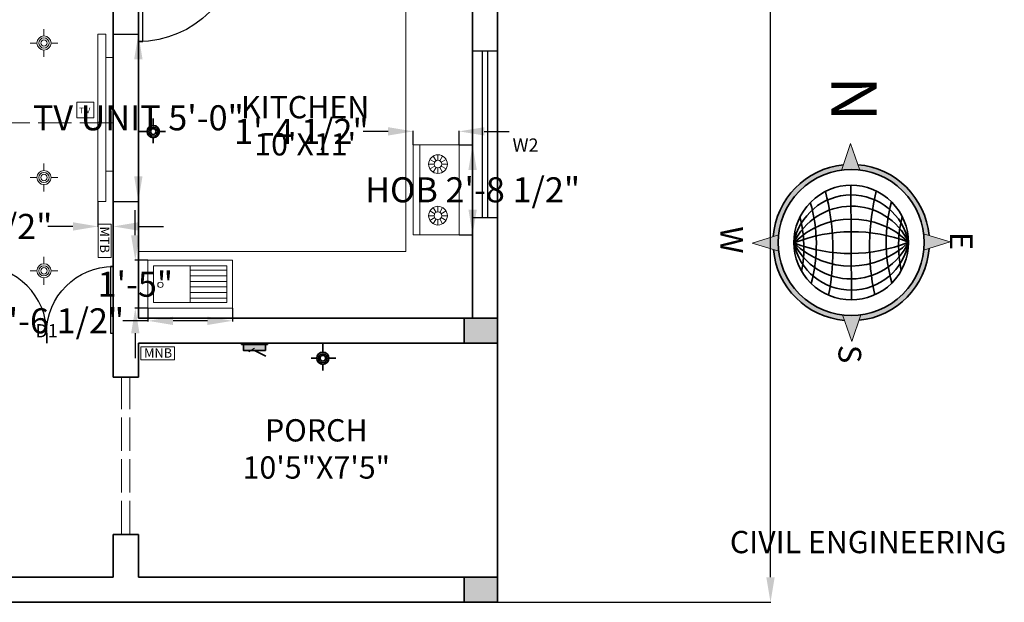
# Model space of a CAD drawing. Units: inches. Extents: x 68 to 1275, y 90 to 1276.
# Tile 5 of 6: x 916 to 1270, y 603 to 813. Entities that reach past the tile are written whole.
import ezdxf

# ---------------------------------------------------------------- set-up
doc = ezdxf.new("R2010")
doc.units = ezdxf.units.IN
doc.header["$MEASUREMENT"] = 0
doc.linetypes.add('ACAD_ISO02W100', pattern=[15, 12, -3])
for name, color, linetype, lineweight in [('A -Elec', 6, 'Continuous', 18), ('A- WALL', 7, 'Continuous', 35), ('A-ANNO-SYMB', 7, 'Continuous', 18), ('A-ANNO-TEXT', 7, 'Continuous', 18), ('A-AREA-IDEN', 7, 'Continuous', 18), ('A-EQPM', 9, 'Continuous', 18), ('A-FLOR-FIXT', 9, 'Continuous', 18), ('A-FLOR-OVHD', 8, 'ACAD_ISO02W100', 13), ('A-TEXT', 7, 'Continuous', 9), ('A-WALL', 7, 'Continuous', 35), ('COLUMN', 150, 'Continuous', 35), ('DIM', 2, 'Continuous', 18), ('DOOR', 15, 'Continuous', 25), ('E-LITE', 6, 'Continuous', 18), ('E-POWR', 1, 'Continuous', 18), ('E-REFR', 8, 'ACAD_ISO02W100', 13), ('Elec', 1, 'Continuous', 35), ('FURN', 163, 'Continuous', 18), ('WINDOW', 17, 'Continuous', 18)]:
    doc.layers.add(name, color=color, linetype=linetype, lineweight=lineweight)
doc.styles.get("Standard").update_dxf_attribs({"font": 'arial.ttf'})
doc.dimstyles.get("Standard").update_dxf_attribs({"dimtxt": 9, "dimasz": 9, "dimexe": 0.18, "dimexo": 0.0625, "dimgap": 0.09, "dimtad": 0, "dimtih": 1, "dimtoh": 1, "dimdec": 1, "dimzin": 0, "dimdsep": 46, "dimlunit": 3, "dimtxsty": 'Standard', "dimcen": 0.09, "dimadec": 0, "dimazin": 0, "dimtfac": 1, "dimtdec": 1, "dimtofl": 0, "dimtmove": 0, "dimatfit": 3, "dimfxl": 1, "dimtolj": 1, "dimtzin": 0, "dimarcsym": 0})

# ---------------------------------------------------------------- blocks, each defined once
blk = doc.blocks.new('*U2')
for p, q in [((0, 0), (-1e-16, -5.999999999999999)), ((40, -6e-16), (40, -6))]:
    blk.add_line(p, q)
blk.add_lwpolyline([(0, 0), (5.6e-15, 40), (1.750000000000007, 40), (1.749999999999998, -7e-16)], close=True)
blk.add_arc((0, 0), 40, 0, 90)
blk = doc.blocks.new('W')
at = {"layer": 'DOOR'}
for p, q in [((91.83571953581463, 414.9514425754601), (100.8357195358146, 414.9514425754601)), ((91.83571953581463, 354.9514425754601), (91.8357195358146, 414.9514425754601)), ((95.33571953581462, 354.9514425754601), (95.33571953581462, 414.9514425754601)), ((97.33571953581463, 354.9514425754601), (97.33571953581463, 414.9514425754601)), ((100.8357195358146, 414.9514425754601), (100.8357195358146, 354.9514425754601)), ((100.8357195358146, 354.9514425754601), (91.83571953581463, 354.9514425754601))]:
    blk.add_line(p, q, dxfattribs=at)
blk = doc.blocks.new('C')
h = blk.add_hatch(color=256)
h.dxf.hatch_style = 1
h.paths.add_polyline_path([(745.8101109123093, 845.9819968167334), (745.8101109123093, 857.9819968167335), (736.8101109123093, 857.9819968167335), (736.8101109123093, 845.9819968167334)])
for p, q in [((745.8101109123093, 857.9819968167335), (736.8101109123093, 857.9819968167335)), ((736.8101109123093, 857.9819968167335), (736.8101109123093, 845.9819968167334)), ((745.8101109123093, 845.9819968167334), (745.8101109123093, 857.9819968167335)), ((736.8101109123093, 845.9819968167334), (745.8101109123093, 845.9819968167334))]:
    blk.add_line(p, q)
blk = doc.blocks.new('TV')
for points in [[(1846.6449218592, 1133.158042881319), (1849.487420558524, 1133.158042881319), (1849.487420558524, 1073.144323226678), (1846.6449218592, 1073.144323226678)], [(1846.6449218592, 1122.373694788675), (1843.999810833538, 1122.373694788675), (1843.999810833538, 1081.482214013656), (1846.6449218592, 1081.482214013656)]]:
    blk.add_lwpolyline(points, close=True)
blk = doc.blocks.new('DIRECTION')
at = {"layer": 'DIM', "ltscale": 35}
h = blk.add_hatch(color=256, dxfattribs=at)
h.dxf.hatch_style = 1
edge = h.paths.add_edge_path()
edge.add_line((2597.24832190935, 2408.269559539512), (2601.856533232682, 2393.62299110183))
edge.add_ellipse((2597.639423319343, 2353.481842285464), major_axis=(28.54028595385228, -28.5402859538523), ratio=0.9999999999827393, start_angle=129.0026750704451, end_angle=135.4089982327699)
edge.add_ellipse((2597.639423319602, 2353.481842285464), major_axis=(-28.54028595291803, -28.54028595291801), ratio=0.999999999985297, start_angle=225.4089982331304, end_angle=231.8159173823239)
edge.add_line((2592.849261358955, 2393.558645959323), (2597.248321909339, 2408.269559539583))
h = blk.add_hatch(color=256, dxfattribs=at)
h.dxf.hatch_style = 1
edge = h.paths.add_edge_path()
edge.add_line((2637.716337406115, 2348.692604170624), (2640.725786551334, 2349.752367405582))
edge.add_ellipse((2597.639423319343, 2353.481842285464), major_axis=(-30.58057945317442, -30.5805794531744), ratio=0.9999999999976388, start_angle=50.166226554127775, end_angle=130.0529151095595, ccw=False)
edge.add_line((2601.533664809112, 2310.41005845266), (2602.42916840349, 2313.404988786752))
edge.add_ellipse((2597.639423319343, 2353.481842285464), major_axis=(-28.54028595136435, -28.54028595136432), ratio=0.9999999999994514, start_angle=51.81532139532596, end_angle=128.185403391547)
edge = h.paths.add_edge_path()
edge.add_line((2593.421895860988, 2313.340737337358), (2594.360152675466, 2310.358877830749))
edge.add_ellipse((2597.639423319343, 2353.481842285464), major_axis=(-30.58057945314276, -30.58057945314273), ratio=0.9999999999967295, start_angle=320.7650813562228, end_angle=400.6513322142664, ccw=False)
edge.add_line((2554.610693956437, 2349.137635932355), (2557.634965847779, 2348.12094433685))
edge.add_ellipse((2597.639423319343, 2353.481842285464), major_axis=(28.54028595137265, -28.54028595137269), ratio=0.9999999999998977, start_angle=232.6325930742551, end_angle=309.0020790836279)
edge = h.paths.add_edge_path()
edge.add_line((2557.562509232831, 2358.271080400352), (2554.553060087694, 2357.211317165394))
edge.add_ellipse((2597.639423319343, 2353.481842285464), major_axis=(-30.58057945310715, -30.58057945310715), ratio=0.9999999999999497, start_angle=230.1666642515818, end_angle=310.0529151095499, ccw=False)
edge.add_line((2593.744852793148, 2396.553596367937), (2592.849261358943, 2393.558645959394))
edge.add_ellipse((2597.639423319343, 2353.481842285464), major_axis=(28.5402859513619, -28.54028595136188), ratio=0.9999999999987931, start_angle=141.8159173820852, end_angle=218.1854033915469)
edge = h.paths.add_edge_path()
edge.add_line((2601.85653323267, 2393.622991101876), (2600.918364535997, 2396.604831790109))
edge.add_ellipse((2597.639423319343, 2353.481842285464), major_axis=(-30.58057945312165, -30.58057945312163), ratio=0.9999999999985156, start_angle=140.765081356223, end_angle=220.6517699116423, ccw=False)
edge.add_line((2640.668152682508, 2357.826048638621), (2637.643880791167, 2358.842740234127))
edge.add_ellipse((2597.639423319343, 2353.481842285464), major_axis=(28.54028595137743, -28.54028595137745), ratio=0.9999999999999049, start_angle=52.63259307425506, end_angle=129.0026750705646)
h = blk.add_hatch(color=256, dxfattribs=at)
h.dxf.hatch_style = 1
edge = h.paths.add_edge_path()
edge.add_ellipse((2597.639423319343, 2353.481842285464), major_axis=(-28.54028595210723, -28.54028595210721), ratio=0.999999999994473, start_angle=308.1854033915466, end_angle=322.6325930742547)
edge.add_line((2557.634965847779, 2348.120944336826), (2542.851706063651, 2353.090740875343))
edge.add_line((2542.851706063651, 2353.090740875343), (2557.562509232831, 2358.271080400328))
h = blk.add_hatch(color=256, dxfattribs=at)
h.dxf.hatch_style = 1
edge = h.paths.add_edge_path()
edge.add_line((2637.643880791167, 2358.84274023415), (2652.427140575295, 2353.87294369554))
edge.add_line((2652.427140575295, 2353.87294369554), (2637.716337406114, 2348.692604170648))
edge.add_ellipse((2597.639423319343, 2353.481842285464), major_axis=(-28.54028595030189, -28.54028595030183), ratio=0.9999999999925798, start_angle=128.1854033915468, end_angle=142.632593074255)
h = blk.add_hatch(color=256, dxfattribs=at)
h.dxf.hatch_style = 1
edge = h.paths.add_edge_path()
edge.add_line((2602.42916840349, 2313.404988786869), (2598.030524729594, 2298.694125031464))
edge.add_line((2598.030524729594, 2298.69412503137), (2593.421895860988, 2313.340737337334))
edge.add_ellipse((2597.639423319602, 2353.481842285464), major_axis=(28.54028595190623, -28.54028595190623), ratio=0.9999999999939888, start_angle=-50.99792091661058, end_angle=-44.59100176735014)
edge.add_ellipse((2597.639423319343, 2353.481842285464), major_axis=(-28.54028595335771, -28.54028595335769), ratio=0.9999999999832972, start_angle=45.40899823301023, end_angle=51.81532139544526)
at = {"layer": 'A- WALL', "ltscale": 35}
blk.add_line((2629.34444276032, 2353.708168156072), (2565.934403878626, 2353.255516414717), dxfattribs=at)
at = {"layer": 'A- WALL', "ltscale": 35, "extrusion": (0, 0, -1)}
for centre, major_axis, ratio, start_param, end_param in [((2597.639423319343, 2353.481842285418), (-30.58057945312132, -30.58057945312131), 0.9999999999987959, 0.8717410831091346, 2.266019187658509), ((2597.639423319343, 2353.481842285418), (28.5402859514277, -28.5402859514277), 0.9999999999973692, 3.919852451189786, 10.20303775836937), ((2597.639423319343, 2353.481842285418), (-30.58057945314268, -30.58057945314266), 0.9999999999988618, 2.432085421867908, 3.826371165679486), ((2597.639423319343, 2353.481842285418), (22.41940544614458, -22.41940544614459), 0.999999999999132, 3.919852451188904, 10.20303775836849), ((2603.542187591361, 2353.523989522555), (22.80466912504525, -22.80466912504527), 0.9999999999934116, 0.9623333078138184, 3.735775406983438), ((2612.505423052941, 2353.587989301701), (-24.76160024723522, -24.76160024723521), 0.9999999999992525, -0.3540869259178678, 1.910602987118144), ((2629.757673802409, 2353.71112763613), (-31.9131967420592, -31.91319674205919), 0.9999999999985343, -0.0006610730671919, 1.55718066820378), ((2599.182585971628, 2445.662182832683), (46.62855256632114, -46.62855256632116), 0.9999999999994293, 0.5735918910566035, 1.030682691728694), ((2678.031679859687, 2354.055802032412), (-61.10857846222063, -61.10857846222057), 0.999999999998412, 0.4026080436482158, 1.153909784551204), ((2517.246998575127, 2352.907900606915), (61.1085784622124, -61.10857846221246), 0.9999999999999429, 5.114997024032398, 5.866298764935286), ((2565.521005037576, 2353.252518252051), (-31.91319674206676, -31.91319674206674), 0.9999999999991755, 3.140929813589933, 4.698771554849301), ((2591.736490906592, 2353.439704278876), (-22.80466912498845, -22.80466912498845), 0.9999999999995747, 2.533131401603469, 5.306573500773075), ((2582.773255331945, 2353.375720337799), (-24.76160024727029, -24.76160024727029), 0.9999999999990459, 2.78750749467719, 5.052197407698938), ((2597.115156409695, 2454.394147896003), (-57.71452300102988, -57.71452300102983), 0.9999999999994852, -1.068719002289636, -0.5124677756952505), ((2597.639423319343, 2353.481842285418), (-30.58057945309982, -30.5805794530998), 0.9999999999997768, -0.7094995924610965, 0.6847785120890495), ((2597.639423319343, 2353.481842285418), (-30.58057945319512, -30.58057945319512), 0.9999999999962719, 4.013333736700001, 5.407619480506816), ((2601.743533004009, 2216.179397968859), (-89.95633825845869, -89.95633825845869), 0.9999999999989515, 2.098588931419211, 2.554035810148795), ((2598.555858798734, 2252.572336165166), (-57.71452300096218, -57.71452300096211), 0.9999999999999362, 2.068987370893696, 2.625238597487658)]:
    blk.add_ellipse(centre, major_axis=major_axis, ratio=ratio, start_param=start_param, end_param=end_param, dxfattribs=at)
at = {"layer": 'A- WALL', "ltscale": 35, "extrusion": (0, 0, -0.9999999999999998)}
for centre, major_axis, ratio, start_param, end_param in [((2599.782951195766, 2490.828885281749), (89.95633825820524, -89.95633825820524), 0.9999999999996148, 0.5732801118446276, 1.028726990569549), ((2600.498417980858, 2261.332926481243), (-46.62855256648622, -46.6285525664862), 0.9999999999990784, 2.096633230266009, 2.553724030937174)]:
    blk.add_ellipse(centre, major_axis=major_axis, ratio=ratio, start_param=start_param, end_param=end_param, dxfattribs=at)
at = {"layer": 'DIM', "ltscale": 35}
for p, q in [((2597.24832190935, 2408.269559539489), (2592.827539238222, 2393.486004940269)), ((2597.24832190935, 2408.269559539489), (2601.879338537261, 2393.550507565663)), ((2542.851706063651, 2353.090740875319), (2557.656003696302, 2358.30400403195)), ((2652.427140575295, 2353.872943695493), (2637.549925830003, 2358.874325760384)), ((2542.851706063651, 2353.090740875319), (2557.728920809025, 2348.089358810546)), ((2652.427140575295, 2353.872943695493), (2637.622842942642, 2348.659680538956)), ((2598.030524729594, 2298.694125031323), (2593.399138912629, 2313.41306084311)), ((2598.030524729594, 2298.694125031323), (2602.450936591041, 2313.477790510296))]:
    blk.add_line(p, q, dxfattribs=at)
at = {"layer": 'A-TEXT', "char_height": 13.629465702112, "width": 273.2349075094469, "attachment_point": 2}
for s, insert in [('{\\fTimes New Roman|b0|i0|c0|p18;\\H0.9233x;E}', (2596.77738151443, 2420.65579489876)), ('{\\fTimes New Roman|b0|i0|c0|p18;\\H0.9233x;S}', (2659.361945474433, 2358.999040747372)), ('{\\fTimes New Roman|b0|i0|c0|p18;\\H0.9233x;W}', (2596.170612003199, 2293.619718441945))]:
    blk.add_mtext(s, dxfattribs=dict(at, insert=insert))
at = {"layer": 'A-TEXT', "insert": (2518.058106811495, 2342.398918831673), "char_height": 27.25893140422401, "width": 546.4698150188938, "attachment_point": 2, "rotation": 179.99999999999997}
blk.add_mtext('{\\fTimes New Roman|b0|i0|c0|p18;\\H0.9233x;N}', dxfattribs=at)
blk = doc.blocks.new('*U28')
blk.add_line((0, 1), (0, -1))
blk = doc.blocks.new('*U29')
at = {"layer": 'FURN', "transparency": 16777216}
blk.add_blockref('*U28', (1741.424228826588, 1059.606151326937), dxfattribs=at)
for p, rotation in [((1739.058647081696, 1057.240569582045), 90), ((1739.375574940783, 1058.423360454491), 59.99999999999999), ((1740.241437954142, 1059.28922346785), 30), ((1742.607019699035, 1059.28922346785), 330.0000000000001), ((1743.472882712394, 1058.423360454491), 300), ((1743.789810571481, 1057.240569582045), 270), ((1739.375574940783, 1056.057778709598), 120), ((1740.241437954142, 1055.191915696239), 150), ((1741.424228826588, 1054.874987837152), 180), ((1742.607019699035, 1055.191915696239), 210), ((1743.472882712394, 1056.057778709598), 240)]:
    blk.add_blockref('*U28', p, dxfattribs=dict(at, rotation=rotation))
blk = doc.blocks.new('*U30')
blk.add_line((0, 1), (0, -1))
blk = doc.blocks.new('*U31')
at = {"layer": 'FURN', "transparency": 16777216}
blk.add_blockref('*U30', (1741.424228826588, 1059.606151326937), dxfattribs=at)
for p, rotation in [((1739.058647081696, 1057.240569582045), 90), ((1739.375574940783, 1058.423360454491), 59.99999999999999), ((1740.241437954142, 1059.28922346785), 30), ((1742.607019699035, 1059.28922346785), 330.0000000000001), ((1743.472882712394, 1058.423360454491), 300), ((1743.789810571481, 1057.240569582045), 270), ((1739.375574940783, 1056.057778709598), 120), ((1740.241437954142, 1055.191915696239), 150), ((1741.424228826588, 1054.874987837152), 180), ((1742.607019699035, 1055.191915696239), 210), ((1743.472882712394, 1056.057778709598), 240)]:
    blk.add_blockref('*U30', p, dxfattribs=dict(at, rotation=rotation))
blk = doc.blocks.new('GAS')
at = {"layer": 'FURN'}
blk.add_line((1734.581424903461, 1063.742262082391), (1766.852210475836, 1063.742262082391), dxfattribs=at)
blk.add_lwpolyline([(1734.581424903461, 1066.149269907321), (1766.852210475836, 1066.149269907321), (1766.852210475836, 1049.6497415827), (1734.581424903461, 1049.6497415827)], close=True, dxfattribs=at)
for centre, radius in [((1741.424228826588, 1057.240569582045), 3.365581744892551), ((1759.93108495299, 1057.240569582045), 3.365581744892551), ((1741.424228826588, 1057.240569582045), 1.365581744892551), ((1759.93108495299, 1057.240569582045), 1.365581744892551)]:
    blk.add_circle(centre, radius, dxfattribs=at)
for name, p in [('*U29', (0, 0)), ('*U31', (18.50685612640154, 0))]:
    blk.add_blockref(name, p, dxfattribs=at)
blk = doc.blocks.new('SINK')
for p, q in [((1691.404714224582, 1155.421202546591), (1708.596639589884, 1155.421202546591)), ((1708.596639589884, 1155.421202546591), (1708.596639589884, 1125.071391182841)), ((1693.404714224582, 1140.246296864716), (1706.596639589884, 1140.246296864716)), ((1695.009100856844, 1140.246296864716), (1695.009100856844, 1127.071391182841)), ((1697.009100856844, 1140.246296864716), (1697.009100856844, 1127.071391182841)), ((1699.009100856844, 1140.246296864716), (1699.009100856844, 1127.071391182841)), ((1701.009100856844, 1140.246296864716), (1701.009100856844, 1127.071391182841)), ((1703.009100856844, 1140.246296864716), (1703.009100856844, 1127.071391182841)), ((1705.009100856844, 1140.246296864716), (1705.009100856844, 1127.071391182841))]:
    blk.add_line(p, q)
for points in [[(1691.404714224582, 1155.421202546591), (1708.596639589884, 1155.421202546591), (1708.596639589884, 1125.071391182841), (1691.404714224582, 1125.071391182841)], [(1693.404714224582, 1153.421202546591), (1706.596639589884, 1153.421202546591), (1706.596639589884, 1127.071391182841), (1693.404714224582, 1127.071391182841)]]:
    blk.add_lwpolyline(points, close=True)
blk.add_circle((1699.780821048727, 1150.931238269399), 0.9650765021387996)
blk = doc.blocks.new('splight')
at = {"layer": 'Elec'}
for p, q in [((4618.165493646445, 527.1595508907546), (4627.57380882646, 527.1595508907546)), ((4622.869651236451, 527.1595508907546), (4622.869651236451, 523.8688723625129)), ((4620.576181531769, 521.5754026578305), (4618.052205676129, 521.5754026578305)), ((4622.869651236451, 519.2819329531479), (4622.869651236451, 517.0346704452847)), ((4625.163120941137, 521.5754026578305), (4627.232633020232, 521.5754026578305))]:
    blk.add_line(p, q, dxfattribs=at)
for radius in [2.293469704682637, 1.668469704682639, 1.043469704682639]:
    blk.add_circle((4622.869651236451, 521.5754026578305), radius, dxfattribs=at)
blk = doc.blocks.new('CIELING')
at = {"layer": 'A -Elec'}
for p, q in [((1070.869500591183, -8395.655580837194), (1070.869500591183, -8391.485789029257)), ((1066.613971407157, -8399.911110021205), (1062.44417959922, -8399.911110021205)), ((1070.869500591183, -8408.33643101315), (1070.869500591183, -8404.166639205214)), ((1075.125029775208, -8399.911110021205), (1079.294821583145, -8399.911110021205))]:
    blk.add_line(p, q, dxfattribs=at)
for radius in [4.255529184009533, 3.095842734009534, 1.936156284009533]:
    blk.add_circle((1070.869500591183, -8399.911110021205), radius, dxfattribs=at)
blk = doc.blocks.new('elec box')
at = {"layer": 'Elec'}
blk.add_hatch(color=256, dxfattribs=at).paths.add_polyline_path([(3828.234962737587, 599.2881263179643), (3828.234962737587, 594.7881263179643), (3844.734962737589, 594.7881263179643), (3844.734962737589, 599.2881263179643)])
for p, q in [((3836.484962737588, 599.2881263179643), (3828.066979685118, 603.4529863194257)), ((3846.10280273742, 594.7881263179643), (3826.830962060027, 594.7881263179643)), ((3826.830962060027, 594.7881263179643), (3826.830962060027, 593.8893551118417)), ((3826.830962060027, 593.8893551118417), (3846.10280273742, 593.8893551118417)), ((3846.10280273742, 593.8893551118417), (3846.10280273742, 594.7881263179643))]:
    blk.add_line(p, q, dxfattribs=at)
blk.add_lwpolyline([(3828.234962737587, 594.7881263179643), (3828.234962737587, 599.2881263179643), (3844.734962737589, 599.2881263179643), (3844.734962737589, 594.7881263179643), (3828.234962737587, 594.7881263179643)], dxfattribs=at)
blk = doc.blocks.new('SWITCHBOARD-ONE-WAY')
blk.add_line((4.634474659967281, 1.72886330620372), (6.643170124125163, 3.124132868275296))
at = {"xscale": 0.480395109260985, "yscale": 0.480395109260985, "zscale": 0.480395109260985}
blk.add_blockref('elec box', (-1838.391242964724, -285.3017071861163), dxfattribs=at)
blk = doc.blocks.new('TV-POINT')
blk.add_lwpolyline([(2.2128117507e-06, 5.568118865895371), (6.100736396045249, 5.568118865895371), (6.100736396045249, -7.01044664311e-05), (2.2128117507e-06, -7.01044664311e-05)], close=True)
at = {"transparency": 33554676}
blk.add_lwpolyline([(2.2128117507e-06, 5.568118865895371), (6.100736396045249, 5.568118865895371), (6.100736396045249, -7.01044664311e-05), (2.2128117507e-06, -7.01044664311e-05)], close=True, dxfattribs=at)
at = {"insert": (0.8393167226115565, 3.647168321161302), "char_height": 2.003474701485161, "attachment_point": 1}
blk.add_mtext('T.V ', dxfattribs=at)
at = {"transparency": 33554676, "insert": (0.8393167226115565, 3.647168321161302), "char_height": 2.003474701485161, "attachment_point": 1}
blk.add_mtext('T.V ', dxfattribs=at)
blk = doc.blocks.new('MAIN-BOARD')
blk.add_lwpolyline([(0.0004361200251424, 4.703133274055858), (12.06279134155943, 4.703133274055858), (12.06279134155943, 0.0003298403245253), (0.0004361200251424, 0.0003298403245253)], close=True)
blk.add_text('MNB', height=3.362765764821897).set_placement((1.14402048200327, 0.7969751531460361))
blk = doc.blocks.new('METER-BOARD')
blk.add_lwpolyline([(0.0004361200251424, 4.702354804303354), (12.06279134155943, 4.702354804303354), (12.06279134155943, -0.0004486294279786), (0.0004361200251424, -0.0004486294279786)], close=True)
blk.add_text('MTB', height=3.362765764821897).set_placement((0.8731259797250459, 0.6934873088445102))
blk = doc.blocks.new('*D67')
at = {"layer": 'Defpoints', "color": 0, "transparency": 16777216}
for p in [(949.6262836938411, 807.4231390285687), (949.6262836938411, 747.4094193739274), (958.6283416420378, 747.4094193739274)]:
    blk.add_point(p, dxfattribs=at)
at = {"layer": 'DIM', "color": 0, "lineweight": -2, "transparency": 16777216}
for p, q in [((949.6887836938411, 807.4231390285687), (958.8083416420376, 807.4231390285687)), ((958.6283416420378, 798.4231390285688), (958.6283416420378, 782.1014360907435)), ((958.6283416420378, 756.4094193739274), (958.6283416420378, 772.731122311753)), ((949.6887836938411, 747.4094193739274), (958.8083416420378, 747.4094193739274))]:
    blk.add_line(p, q, dxfattribs=at)
at = {"layer": 'DIM', "color": 0, "transparency": 16777216}
for points in [[(957.1283416420378, 798.4231390285688), (960.1283416420378, 798.4231390285688), (958.6283416420378, 807.4231390285687)], [(957.1283416420378, 756.4094193739274), (960.1283416420379, 756.4094193739274), (958.6283416420378, 747.4094193739274)]]:
    blk.add_solid(points, dxfattribs=at)
at = {"layer": 'DIM', "color": 0, "transparency": 16777216, "insert": (958.6283416420378, 777.4162792012476), "char_height": 9, "attachment_point": 5}
blk.add_mtext('\\A1;TV UNIT 5\'-0"', dxfattribs=at)
blk = doc.blocks.new('*D68')
at = {"layer": 'Defpoints', "color": 0, "transparency": 16777216}
for p in [(944.1386739688546, 747.4094193739272), (949.6262836938406, 747.4094193739272), (944.1386739688546, 738.407361425731)]:
    blk.add_point(p, dxfattribs=at)
at = {"layer": 'DIM', "color": 0, "lineweight": -2, "transparency": 16777216}
for p, q in [((944.1386739688546, 747.3469193739272), (944.1386739688546, 738.2273614257311)), ((949.6262836938406, 747.3469193739272), (949.6262836938406, 738.2273614257311)), ((935.1386739688546, 738.407361425731), (926.1386739688546, 738.407361425731)), ((958.6262836938406, 738.407361425731), (967.6262836938406, 738.407361425731))]:
    blk.add_line(p, q, dxfattribs=at)
at = {"layer": 'DIM', "color": 0, "transparency": 16777216}
for points in [[(935.1386739688546, 739.9073614257311), (935.1386739688546, 736.9073614257311), (944.1386739688546, 738.407361425731)], [(958.6262836938406, 739.9073614257311), (958.6262836938406, 736.9073614257311), (949.6262836938406, 738.407361425731)]]:
    blk.add_solid(points, dxfattribs=at)
at = {"layer": 'DIM', "color": 0, "transparency": 16777216, "insert": (903.6008567792229, 738.407361425731), "char_height": 9, "attachment_point": 5}
blk.add_mtext('\\A1;0\'-5 1/2"', dxfattribs=at)
blk = doc.blocks.new('*D69')
at = {"layer": 'Defpoints', "color": 0, "transparency": 16777216}
for p in [(962.0814133719534, 709.0733946794592), (992.4312247357036, 709.0733946794592), (962.0814133719534, 704.5209229748966)]:
    blk.add_point(p, dxfattribs=at)
at = {"layer": 'DIM', "color": 0, "lineweight": -2, "transparency": 16777216}
for p, q in [((962.0814133719534, 709.010894679459), (962.0814133719534, 704.3409229748966)), ((992.4312247357036, 709.010894679459), (992.4312247357036, 704.3409229748966)), ((962.0814133719534, 704.5209229748966), (953.0814133719534, 704.5209229748966)), ((983.4312247357036, 704.5209229748966), (971.0814133719534, 704.5209229748966))]:
    blk.add_line(p, q, dxfattribs=at)
at = {"layer": 'DIM', "color": 0, "transparency": 16777216}
for points in [[(971.0814133719534, 706.0209229748966), (971.0814133719534, 703.0209229748966), (962.0814133719534, 704.5209229748966)], [(983.4312247357036, 706.0209229748966), (983.4312247357036, 703.0209229748966), (992.4312247357036, 704.5209229748966)]]:
    blk.add_solid(points, dxfattribs=at)
at = {"layer": 'DIM', "color": 0, "transparency": 16777216, "insert": (914.1459154183381, 704.5209229748966), "char_height": 9, "attachment_point": 5}
blk.add_mtext('\\A1;SINK 2\'-6 1/2"', dxfattribs=at)
blk = doc.blocks.new('*D70')
at = {"layer": 'Defpoints', "color": 0, "transparency": 16777216}
for p in [(957.5289416673916, 726.2653200447614), (962.0814133719539, 726.2653200447614), (962.0814133719539, 709.0733946794594)]:
    blk.add_point(p, dxfattribs=at)
at = {"layer": 'DIM', "color": 0, "lineweight": -2, "transparency": 16777216}
for p, q in [((957.5289416673916, 735.2653200447614), (957.5289416673916, 744.2653200447614)), ((962.0189133719538, 726.2653200447614), (957.3489416673917, 726.2653200447614)), ((962.0189133719538, 709.0733946794594), (957.3489416673917, 709.0733946794594)), ((957.5289416673916, 700.0733946794594), (957.5289416673916, 691.0733946794594))]:
    blk.add_line(p, q, dxfattribs=at)
at = {"layer": 'DIM', "color": 0, "transparency": 16777216}
for points in [[(956.0289416673917, 735.2653200447614), (959.0289416673916, 735.2653200447614), (957.5289416673916, 726.2653200447614)], [(956.0289416673917, 700.0733946794594), (959.0289416673916, 700.0733946794594), (957.5289416673916, 709.0733946794594)]]:
    blk.add_solid(points, dxfattribs=at)
at = {"layer": 'DIM', "color": 0, "transparency": 16777216, "insert": (957.5289416673916, 717.66935736211), "char_height": 9, "attachment_point": 5}
blk.add_mtext('\\A1;1\'-5"', dxfattribs=at)
blk = doc.blocks.new('*D71')
at = {"layer": 'Defpoints', "color": 0, "transparency": 16777216}
for p in [(1073.789909938414, 767.698910965495), (1078.630527774271, 767.698910965495), (1073.789909938414, 735.4281253931201)]:
    blk.add_point(p, dxfattribs=at)
at = {"layer": 'DIM', "color": 0, "lineweight": -2, "transparency": 16777216}
for p, q in [((1073.852409938414, 767.698910965495), (1078.810527774271, 767.698910965495)), ((1078.630527774271, 758.698910965495), (1078.630527774271, 756.3100666104126)), ((1078.630527774271, 744.4281253931201), (1078.630527774271, 746.8169697482026)), ((1073.852409938414, 735.4281253931201), (1078.810527774271, 735.4281253931201))]:
    blk.add_line(p, q, dxfattribs=at)
at = {"layer": 'DIM', "color": 0, "transparency": 16777216}
for points in [[(1077.130527774271, 758.698910965495), (1080.13052777427, 758.698910965495), (1078.630527774271, 767.698910965495)], [(1077.130527774271, 744.4281253931201), (1080.13052777427, 744.4281253931201), (1078.630527774271, 735.4281253931201)]]:
    blk.add_solid(points, dxfattribs=at)
at = {"layer": 'DIM', "color": 0, "transparency": 16777216, "insert": (1078.630527774271, 751.5635181793072), "char_height": 9, "attachment_point": 5}
blk.add_mtext('\\A1;HOB 2\'-8 1/2"', dxfattribs=at)
blk = doc.blocks.new('*D72')
at = {"layer": 'Defpoints', "color": 0, "transparency": 16777216}
for p in [(1057.290381613793, 772.5395288013511), (1057.290381613793, 767.6989109654947), (1073.789909938414, 767.6989109654947)]:
    blk.add_point(p, dxfattribs=at)
at = {"layer": 'DIM', "color": 0, "lineweight": -2, "transparency": 16777216}
for p, q in [((1048.290381613792, 772.5395288013511), (1039.290381613793, 772.5395288013511)), ((1057.290381613793, 767.7614109654947), (1057.290381613793, 772.719528801351)), ((1073.789909938414, 767.7614109654947), (1073.789909938414, 772.719528801351)), ((1082.789909938414, 772.5395288013511), (1091.789909938414, 772.5395288013511))]:
    blk.add_line(p, q, dxfattribs=at)
at = {"layer": 'DIM', "color": 0, "transparency": 16777216}
for points in [[(1048.290381613792, 774.0395288013511), (1048.290381613792, 771.0395288013511), (1057.290381613793, 772.5395288013511)], [(1082.789909938414, 774.0395288013511), (1082.789909938414, 771.0395288013511), (1073.789909938414, 772.5395288013511)]]:
    blk.add_solid(points, dxfattribs=at)
at = {"layer": 'DIM', "color": 0, "transparency": 16777216, "insert": (1017.176166061269, 772.5395288013511), "char_height": 9, "attachment_point": 5}
blk.add_mtext('\\A1;1\'-4 1/2"', dxfattribs=at)
blk = doc.blocks.new('*D113')
at = {"layer": 'Defpoints', "color": 0, "transparency": 16777216}
for p in [(1087.626284, 1232.468609), (1185.576284000001, 1232.468609), (1087.626284, 603.4686090000002)]:
    blk.add_point(p, dxfattribs=at)
at = {"layer": 'DIM', "color": 0, "lineweight": -2, "transparency": 16777216}
for p, q in [((1087.688784, 1232.468609), (1185.756284000001, 1232.468609)), ((1185.576284000001, 1223.468609), (1185.576284000001, 922.6537658894956)), ((1185.576284000001, 612.4686090000002), (1185.576284000001, 913.2834521105051)), ((1087.688784, 603.4686090000002), (1185.756284000001, 603.4686090000002))]:
    blk.add_line(p, q, dxfattribs=at)
at = {"layer": 'DIM', "color": 0, "transparency": 16777216}
for points in [[(1184.076284000001, 1223.468609), (1187.076284000001, 1223.468609), (1185.576284000001, 1232.468609)], [(1184.076284000001, 612.4686090000002), (1187.076284000001, 612.4686090000002), (1185.576284000001, 603.4686090000002)]]:
    blk.add_solid(points, dxfattribs=at)
at = {"layer": 'DIM', "color": 0, "transparency": 16777216, "insert": (1185.576284000001, 917.9686089999998), "char_height": 9, "attachment_point": 5}
blk.add_mtext('\\A1;52\'-5"', dxfattribs=at)

msp = doc.modelspace()

# ---------------------------------------------------------------- linework, layer by layer
at = {"layer": 'A-FLOR-FIXT'}
for p in [(1054.626283693841, 837.4686089321809), (958.6262836938411, 729.4686089321808)]:
    msp.add_line(p, (1054.626283693841, 729.4686089321808), dxfattribs=at)
at = {"layer": 'A-FLOR-OVHD'}
for p, q in [((952.6262836938411, 627.8603246065964), (952.6262836938411, 684.3088251010706)), ((955.626283693841, 627.8603246065964), (955.626283693841, 684.3088251010706))]:
    msp.add_line(p, q, dxfattribs=at)
at = {"layer": 'A-WALL'}
for p, q in [((1087.626283693841, 941.4686089321808), (1087.626283693841, 696.4686089321808)), ((949.6262836938411, 846.4686089321808), (949.6262836938411, 705.4686089321807)), ((958.6262836938411, 837.4686089321809), (958.6262836938411, 705.4686089321807)), ((1078.626283693841, 837.4686089321809), (1078.626283693841, 705.4686089321807)), ((949.6262836938411, 696.4686089321808), (949.6262836938411, 705.4686089321807)), ((958.6262836938411, 705.4686089321807), (1078.626283693841, 705.4686089321807)), ((949.6262836938411, 684.3088251010706), (949.6262836938411, 696.4686089321808)), ((958.6262836938411, 696.4686089321808), (1087.626283693841, 696.4686089321808)), ((958.6262836938411, 684.3088251010706), (958.6262836938411, 696.4686089321808)), ((1087.626283693841, 603.4686089321808), (1087.626283693841, 696.4686089321808)), ((949.6262836938411, 684.3088251010706), (958.6262836938411, 684.3088251010706)), ((949.6262836938411, 612.4686089321808), (949.6262836938411, 627.8603246065964)), ((958.6262836938411, 627.8603246065964), (949.6262836938411, 627.8603246065964)), ((958.6262836938411, 612.4686089321808), (958.6262836938411, 627.8603246065964)), ((727.6262836938411, 612.4686089321808), (949.6262836938411, 612.4686089321808)), ((958.6262836938411, 612.4686089321808), (1087.626283693841, 612.4686089321808)), ((718.6262836938411, 603.4686089321808), (1087.626283693841, 603.4686089321808))]:
    msp.add_line(p, q, dxfattribs=at)
at = {"layer": 'E-REFR'}
msp.add_line((727.6262836938411, 775.5635401615964), (949.6262836938411, 775.5635401615964), dxfattribs=at)

# ---------------------------------------------------------------- block references
at = {"layer": 'A-ANNO-SYMB', "xscale": 0.648641096179051, "yscale": 0.648641096179051, "zscale": 0.648641096179051, "rotation": 270}
msp.add_blockref('DIRECTION', (-312.0034923453442, 2417.554004507394), dxfattribs=at)
at = {"layer": 'A-EQPM'}
for name, p, rotation in [('TV', (2793.626094527379, 1880.567462255246), 180), ('GAS', (2123.439651521114, -999.1532995103412), 90)]:
    msp.add_blockref(name, p, dxfattribs=dict(at, rotation=rotation))
at = {"layer": 'A-FLOR-FIXT', "rotation": 89.99999999999999}
msp.add_blockref('SINK', (2117.502615918544, -982.331319545123), dxfattribs=at)
at = {"layer": 'COLUMN', "rotation": 270}
for p in [(229.6442868771078, 1442.27871984449), (229.6442868771077, 1349.27871984449)]:
    msp.add_blockref('C', p, dxfattribs=at)
at = {"layer": 'DOOR', "xscale": -0.9060456833541303, "yscale": 0.9060456833541303, "zscale": 0.9060456833541303, "rotation": 180}
msp.add_blockref('*U2', (958.6262836938411, 841.0323348320559), dxfattribs=at)
at = {"layer": 'DOOR'}
for p, xscale, yscale, zscale in [((901.6262836938411, 700.0825684476132), 0.6023265859053817, 0.6023265859053817, 0.6023265859053817), ((949.6262836938411, 700.0594686443264), -0.5984766186909284, 0.5984766186909284, 0.5984766186909284)]:
    msp.add_blockref('*U2', p, dxfattribs=dict(at, xscale=xscale, yscale=yscale, zscale=zscale))
at = {"layer": 'E-LITE', "transparency": 33554676, "xscale": 0.5930528030907906, "yscale": 0.5930528030907906, "zscale": 0.5930528030907906}
for p in [(289.6667483386187, 5785.855102200456), (289.6667483386186, 5737.560666567257), (289.6667483386185, 5704.070193875034)]:
    msp.add_blockref('CIELING', p, dxfattribs=at)
at = {"layer": 'E-LITE', "xscale": -0.9617510087435096, "yscale": 0.9617510087435096, "zscale": 0.9617510087390623}
for p, rotation in [((1465.622513531819, 5218.52377952538), 89.99999999999976), ((5470.914053965565, 189.4723790942011), 359.9999999999997)]:
    msp.add_blockref('splight', p, dxfattribs=dict(at, rotation=rotation))
at = {"layer": 'E-POWR'}
for name, p in [('TV-POINT', (936.551448719158, 777.430527842383)), ('MAIN-BOARD', (959.548275551138, 690.5170294169185))]:
    msp.add_blockref(name, p, dxfattribs=at)
for name, p, rotation in [('METER-BOARD', (944.210880014749, 739.2618495944421), 270.0000000000005), ('SWITCHBOARD-ONE-WAY', (1004.945216716659, 696.4684433839539), 180)]:
    msp.add_blockref(name, p, dxfattribs=dict(at, rotation=rotation))
at = {"layer": 'WINDOW'}
msp.add_blockref('W', (986.7905641580264, 386.5171663567208), dxfattribs=at)

# ---------------------------------------------------------------- texts
at = {"layer": 'A-ANNO-TEXT', "width": 20.39887023007676, "attachment_point": 5}
for s, insert, char_height in [('{\\fTimes New Roman|b0|i0|c0|p18;\\H0.8x;W2}', (1097.643488395882, 767.6056201989016), 5.953092231351539), ('{\\fTimes New Roman|b0|i0|c0|p18;\\H0.8x;D1}', (925.7037571773704, 700.9491573878294), 5.953076141217599)]:
    msp.add_mtext(s, dxfattribs=dict(at, insert=insert, char_height=char_height))
at = {"layer": 'A-ANNO-TEXT', "insert": (1220.666804533313, 629.1012558852271), "char_height": 8, "attachment_point": 2}
msp.add_mtext_dynamic_manual_height_columns('CIVIL ENGINEERING', width=128.8568059801491, gutter_width=1, heights=[0], dxfattribs=at)
at = {"layer": 'A-AREA-IDEN', "char_height": 8, "attachment_point": 2}
for s, insert in [("KITCHEN\\P10'X11'", (1018.51541272249, 785.2247260609533)), ('PORCH\\P10\'5"X7\'5"', (1022.52005010476, 669.2079792889501))]:
    msp.add_mtext_dynamic_manual_height_columns(s, width=128.8568059801491, gutter_width=1, heights=[0], dxfattribs=dict(at, insert=insert))

# ---------------------------------------------------------------- dimensions: what is measured, and where the dimension line sits
at = {"layer": 'DIM'}
for base, p1, p2, angle, picture, middle in [((1185.576284000001, 1232.468609), (1087.626284, 603.468609), (1087.626284, 1232.468609), 90, '*D113', (1185.576284000001, 917.9686089999998)), ((1057.290381613793, 772.5395288013511), (1073.789909938414, 767.6989109654947), (1057.290381613793, 767.6989109654947), 180, '*D72', (1017.176166061269, 772.5395288013511)), ((944.1386739688546, 738.407361425731), (949.6262836938406, 747.4094193739272), (944.1386739688546, 747.4094193739272), 180, '*D68', (903.6008567792229, 738.407361425731)), ((957.5289416673916, 726.2653200447614), (962.0814133719534, 709.0733946794592), (962.0814133719534, 726.2653200447612), 90, '*D70', (957.5289416673916, 717.66935736211))]:
    dim = msp.add_linear_dim(base=base, p1=p1, p2=p2, angle=angle, dimstyle='Standard', override={"dimdec": 1, "dimlfac": 1, "dimrnd": 0, "dimzin": 1, "dimdsep": 46, "dimlunit": 4, "dimfrac": 2}, dxfattribs=at)
    dim.commit()
    dim.dimension.update_dxf_attribs({"geometry": picture, "text_midpoint": middle})
for base, p1, p2, angle, text, picture, middle in [((958.6283416420378, 747.4094193739274), (949.6262836938406, 807.4231390285682), (949.6262836938406, 747.4094193739272), 270, 'TV UNIT <>', '*D67', (958.6283416420378, 777.4162792012476)), ((1078.630527774271, 767.698910965495), (1073.789909938414, 735.4281253931199), (1073.789909938414, 767.6989109654947), 90, 'HOB <>', '*D71', (1078.630527774271, 751.5635181793072)), ((962.0814133719534, 704.5209229748966), (992.4312247357036, 709.0733946794592), (962.0814133719534, 709.0733946794592), 180, 'SINK <>', '*D69', (914.1459154183381, 704.5209229748966))]:
    dim = msp.add_linear_dim(base=base, p1=p1, p2=p2, angle=angle, text=text, dimstyle='Standard', override={"dimdec": 1, "dimlfac": 1, "dimrnd": 0, "dimzin": 1, "dimdsep": 46, "dimlunit": 4, "dimfrac": 2}, dxfattribs=at)
    dim.commit()
    dim.dimension.update_dxf_attribs({"geometry": picture, "text_midpoint": middle})

doc.saveas('drawing.dxf')
